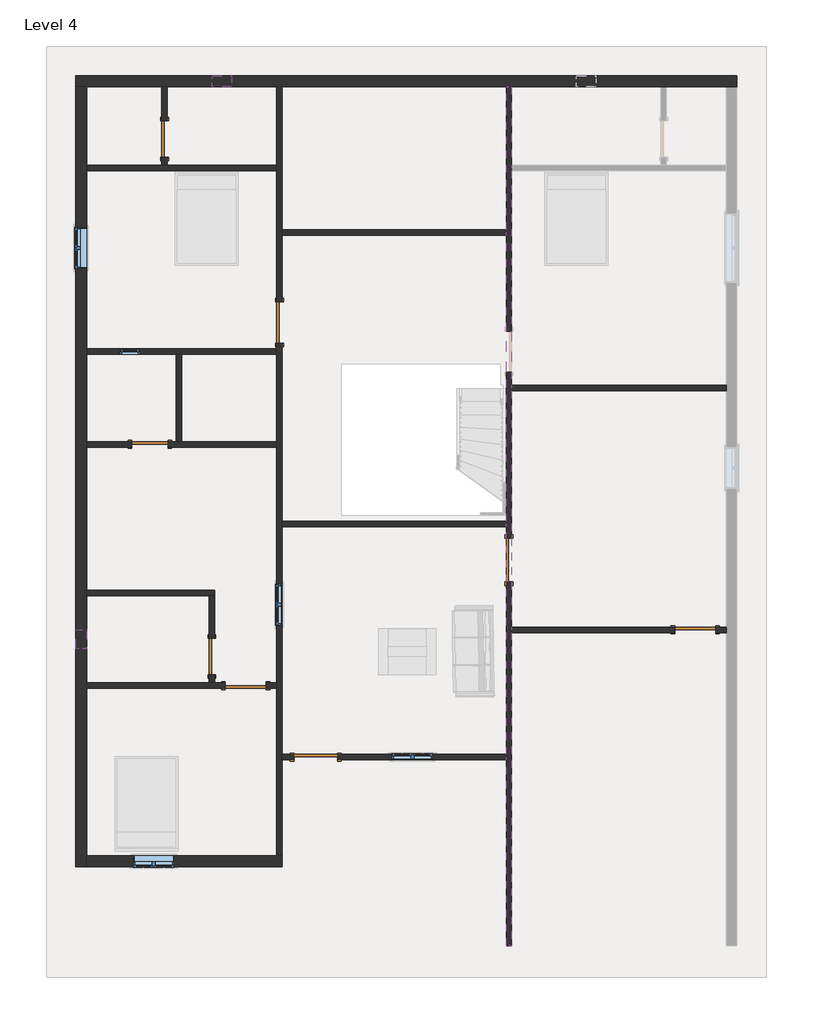
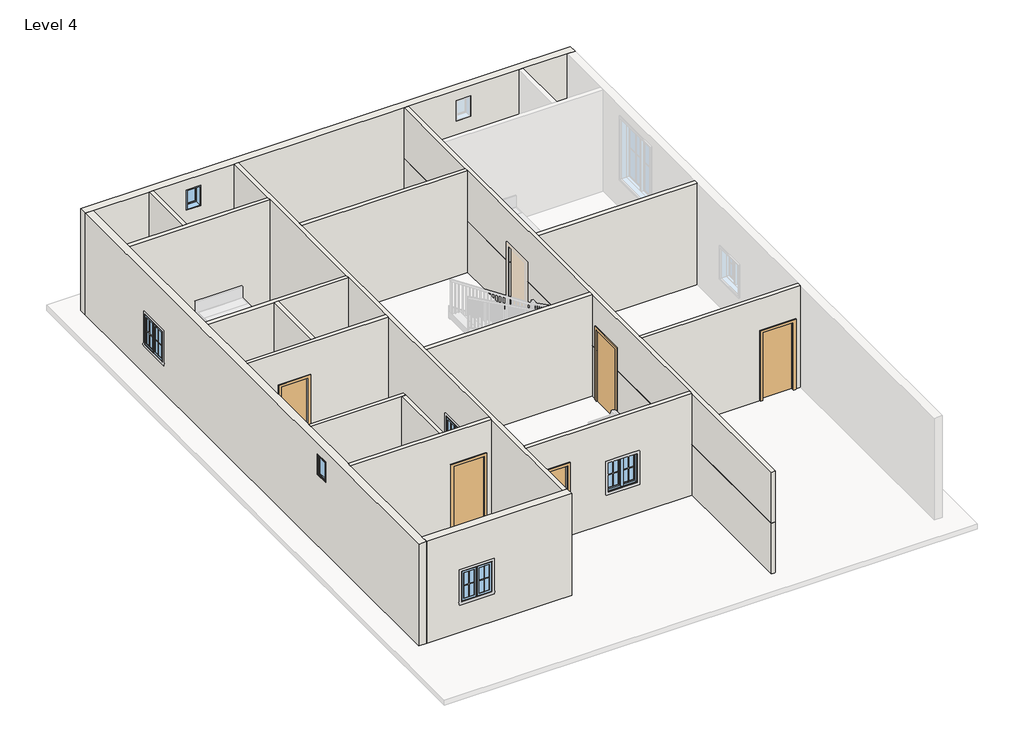
# One storey, part 1 of 3: 19 walls, 8 doors, 7 windows.
"""IFC4 building model written with IfcOpenShell, lengths in millimetres."""

from ifc_helpers import new_model, si_unit, frame, origin, place, context, project, spatial, polyline, outline, extrude, faceted_brep, transform, mapped, element, save
from components import door_f2b275c1, door_d8f5dbb5, door_825b8444, door_c29894e6, door_305aa2a5, window_aa618e30, window_a10b4202, window_339605e1, window_a598f463

model = new_model("IFC4")

# Units and contexts
model_context = context("Model", 3, world=origin())
ifc_project = project(units=[si_unit("LENGTHUNIT", "METRE", prefix="MILLI")], contexts=[model_context])

# Site, building, storey
site = spatial("IfcSite", under=ifc_project)
building = spatial("IfcBuilding", under=site)
storey = spatial("IfcBuildingStorey", under=building, Name="Level 4", Elevation=6400.8)

# Doors
placement = place(None, origin())
door_shape = door_f2b275c1(model_context)
element("IfcDoor", 1, ObjectType="Single-Flush : 30\" x 80\"", at=placement, inside=storey, context=model_context, shape_type="MappedRepresentation", body=[
    mapped(door_shape, transform((-5639.8561469, 9100.7522623, 6400.8), x_axis=(0.0, -1.0, 0.0), y_axis=(1.0, 0.0, 0.0), z_axis=(0.0, 0.0, 1.0))),
])
element("IfcDoor", 2, ObjectType="Single-Flush : 30\" x 80\"", at=placement, inside=storey, context=model_context, shape_type="MappedRepresentation", body=[
    mapped(door_shape, transform((-4646.033646, -1745.0477377, 6400.8), x_axis=(0.0, -1.0, 0.0), y_axis=(1.0, 0.0, 0.0), z_axis=(0.0, 0.0, 1.0))),
])
door_2_shape = door_d8f5dbb5(model_context)
element("IfcDoor", 3, ObjectType="Single-Flush : 30\" x 80\"", at=placement, inside=storey, context=model_context, shape_type="MappedRepresentation", body=[
    mapped(door_2_shape, transform((-5947.8915084, 2699.9522623, 6400.8), x_axis=(1.0, 0.0, 0.0), y_axis=(0.0, 1.0, 0.0), z_axis=(0.0, 0.0, 1.0))),
])
door_3_shape = door_825b8444(model_context)
element("IfcDoor", 4, ObjectType="Single-Flush : 34\" x 80\"", at=placement, inside=storey, context=model_context, shape_type="MappedRepresentation", body=[
    mapped(door_3_shape, transform((-3230.0915084, 5252.6522623, 6400.8), x_axis=(0.0, -1.0, 0.0), y_axis=(1.0, 0.0, 0.0), z_axis=(0.0, 0.0, 1.0))),
])
element("IfcDoor", 5, ObjectType="Single-Flush : 34\" x 80\"", at=placement, inside=storey, context=model_context, shape_type="MappedRepresentation", body=[
    mapped(door_3_shape, transform((-3938.0625772, -2354.6477377, 6400.8), x_axis=(1.0, 0.0, 0.0), y_axis=(0.0, 1.0, 0.0), z_axis=(0.0, 0.0, 1.0))),
])
door_4_shape = door_c29894e6(model_context)
element("IfcDoor", 6, ObjectType="Single-Flush : 34\" x 80\"", at=placement, inside=storey, context=model_context, shape_type="MappedRepresentation", body=[
    mapped(door_4_shape, transform((5488.4584916, -1186.2477377, 6400.8), x_axis=(1.0, 0.0, 0.0), y_axis=(0.0, 1.0, 0.0), z_axis=(0.0, 0.0, 1.0))),
])
door_5_shape = door_305aa2a5(model_context)
element("IfcDoor", 7, ObjectType="Single-Flush : 36\" x 84\"", at=placement, inside=storey, context=model_context, shape_type="MappedRepresentation", body=[
    mapped(door_5_shape, transform((1583.2084916, 274.2522623, 6400.8), x_axis=(0.0, -1.0, 0.0), y_axis=(1.0, 0.0, 0.0), z_axis=(0.0, 0.0, 1.0))),
])
element("IfcDoor", 8, ObjectType="Single-Flush : 36\" x 84\"", at=placement, inside=storey, context=model_context, shape_type="MappedRepresentation", body=[
    mapped(door_5_shape, transform((-2468.0915084, -3853.2477377, 6400.8), x_axis=(-1.0, 0.0, 0.0), y_axis=(0.0, -1.0, 0.0), z_axis=(0.0, 0.0, 1.0))),
])

# Walls
element("IfcWall", 9, ObjectType="9\"", at=placement, inside=storey, context=model_context, shape_type="Brep", body=[
    faceted_brep([(-7503.6415084, 10199.3022623, 6400.8), (-7275.0415084, 10199.3022623, 6400.8), (-5697.0061469, 10199.3022623, 6400.8), (-5582.7061469, 10199.3022623, 6400.8), (-3287.2415084, 10199.3022623, 6400.8), (-3172.9415084, 10199.3022623, 6400.8), (1526.0584916, 10199.3022623, 6400.8), (1640.3584916, 10199.3022623, 6400.8), (4770.1866507, 10199.3022623, 6400.8), (4884.4866507, 10199.3022623, 6400.8), (6136.1584916, 10199.3022623, 6400.8), (6364.7584916, 10199.3022623, 6400.8), (6364.7584916, 10199.3022623, 9448.8), (6136.1584916, 10199.3022623, 9448.8), (4884.4866507, 10199.3022623, 9448.8), (4770.1866507, 10199.3022623, 9448.8), (1640.3584916, 10199.3022623, 9448.8), (1526.0584916, 10199.3022623, 9448.8), (-3172.9415084, 10199.3022623, 9448.8), (-3287.2415084, 10199.3022623, 9448.8), (-5582.7061469, 10199.3022623, 9448.8), (-5697.0061469, 10199.3022623, 9448.8), (-7275.0415084, 10199.3022623, 9448.8), (-7503.6415084, 10199.3022623, 9448.8), (-4231.7738276, 10199.3022623, 9144.0), (-4231.7738276, 10199.3022623, 8534.4), (-4638.1738276, 10199.3022623, 8534.4), (-4638.1738276, 10199.3022623, 9144.0), (3408.4725711, 10199.3022623, 9144.0), (3408.4725711, 10199.3022623, 8534.4), (3002.0725711, 10199.3022623, 8534.4), (3002.0725711, 10199.3022623, 9144.0), (-7503.6415084, 10427.9022623, 6400.8), (-7503.6415084, 10427.9022623, 9448.8), (6364.7584916, 10427.9022623, 9448.8), (6364.7584916, 10427.9022623, 6400.8), (-4231.7738276, 10427.9022623, 9144.0), (-4638.1738276, 10427.9022623, 9144.0), (-4638.1738276, 10427.9022623, 8534.4), (-4231.7738276, 10427.9022623, 8534.4), (3408.4725711, 10427.9022623, 9144.0), (3002.0725711, 10427.9022623, 9144.0), (3002.0725711, 10427.9022623, 8534.4), (3408.4725711, 10427.9022623, 8534.4)], [[[0, 1, 2, 3, 4, 5, 6, 7, 8, 9, 10, 11, 12, 13, 14, 15, 16, 17, 18, 19, 20, 21, 22, 23], [24, 25, 26, 27], [28, 29, 30, 31]], [[32, 33, 34, 35], [36, 37, 38, 39], [40, 41, 42, 43]], [[11, 10, 9, 8, 7, 6, 5, 4, 3, 2, 1, 0, 32, 35]], [[12, 11, 35, 34]], [[25, 24, 36, 39]], [[26, 25, 39, 38]], [[27, 26, 38, 37]], [[24, 27, 37, 36]], [[29, 28, 40, 43]], [[30, 29, 43, 42]], [[31, 30, 42, 41]], [[28, 31, 41, 40]], [[23, 22, 21, 20, 19, 18, 17, 16, 15, 14, 13, 12, 34, 33]], [[0, 23, 33, 32]]]),
])
element("IfcWall", 10, ObjectType="9\"", at=placement, inside=storey, context=model_context, shape_type="Brep", body=[
    faceted_brep([(-7503.6415084, 10199.3022623, 6400.8), (-7503.6415084, -6145.5977377, 6400.8), (-7503.6415084, -6145.5977377, 9448.8), (-7503.6415084, 10199.3022623, 9448.8), (-7503.6415084, -1179.8977377, 9144.0), (-7503.6415084, -1586.2977377, 9144.0), (-7503.6415084, -1586.2977377, 8534.4), (-7503.6415084, -1179.8977377, 8534.4), (-7503.6415084, 7246.5522623, 8229.6), (-7503.6415084, 6382.9522623, 8229.6), (-7503.6415084, 6382.9522623, 7315.2), (-7503.6415084, 7246.5522623, 7315.2), (-7275.0415084, 10199.3022623, 6400.8), (-7275.0415084, 10199.3022623, 9448.8), (-7275.0415084, 8548.3022623, 9448.8), (-7275.0415084, 8434.0022623, 9448.8), (-7275.0415084, 4700.2022623, 9448.8), (-7275.0415084, 4585.9022623, 9448.8), (-7275.0415084, 2757.1022623, 9448.8), (-7275.0415084, 2642.8022623, 9448.8), (-7275.0415084, -354.3977377, 9448.8), (-7275.0415084, -468.6977377, 9448.8), (-7275.0415084, -2297.4977377, 9448.8), (-7275.0415084, -2411.7977377, 9448.8), (-7275.0415084, -5916.9977377, 9448.8), (-7275.0415084, -6145.5977377, 9448.8), (-7275.0415084, -6145.5977377, 6400.8), (-7275.0415084, -5916.9977377, 6400.8), (-7275.0415084, -2411.7977377, 6400.8), (-7275.0415084, -2297.4977377, 6400.8), (-7275.0415084, -468.6977377, 6400.8), (-7275.0415084, -354.3977377, 6400.8), (-7275.0415084, 2642.8022623, 6400.8), (-7275.0415084, 2757.1022623, 6400.8), (-7275.0415084, 4585.9022623, 6400.8), (-7275.0415084, 4700.2022623, 6400.8), (-7275.0415084, 8434.0022623, 6400.8), (-7275.0415084, 8548.3022623, 6400.8), (-7275.0415084, -1179.8977377, 9144.0), (-7275.0415084, -1179.8977377, 8534.4), (-7275.0415084, -1586.2977377, 8534.4), (-7275.0415084, -1586.2977377, 9144.0), (-7275.0415084, 7246.5522623, 8229.6), (-7275.0415084, 7246.5522623, 7315.2), (-7275.0415084, 6382.9522623, 7315.2), (-7275.0415084, 6382.9522623, 8229.6)], [[[0, 1, 2, 3], [4, 5, 6, 7], [8, 9, 10, 11]], [[12, 13, 14, 15, 16, 17, 18, 19, 20, 21, 22, 23, 24, 25, 26, 27, 28, 29, 30, 31, 32, 33, 34, 35, 36, 37], [38, 39, 40, 41], [42, 43, 44, 45]], [[1, 0, 12, 37, 36, 35, 34, 33, 32, 31, 30, 29, 28, 27, 26]], [[2, 1, 26, 25]], [[39, 38, 4, 7]], [[40, 39, 7, 6]], [[41, 40, 6, 5]], [[38, 41, 5, 4]], [[43, 42, 8, 11]], [[44, 43, 11, 10]], [[45, 44, 10, 9]], [[42, 45, 9, 8]], [[3, 2, 25, 24, 23, 22, 21, 20, 19, 18, 17, 16, 15, 14, 13]], [[0, 3, 13, 12]]]),
])
element("IfcWall", 11, ObjectType="9\"", at=placement, inside=storey, context=model_context, shape_type="Brep", body=[
    faceted_brep([(-7275.0415084, -6145.5977377, 6400.8), (-3172.9415084, -6145.5977377, 6400.8), (-3172.9415084, -6145.5977377, 9448.8), (-7275.0415084, -6145.5977377, 9448.8), (-6297.1415084, -6145.5977377, 8229.6), (-5433.5415084, -6145.5977377, 8229.6), (-5433.5415084, -6145.5977377, 7315.2), (-6297.1415084, -6145.5977377, 7315.2), (-7275.0415084, -5916.9977377, 6400.8), (-7275.0415084, -5916.9977377, 9448.8), (-3287.2415084, -5916.9977377, 9448.8), (-3172.9415084, -5916.9977377, 9448.8), (-3172.9415084, -5916.9977377, 6400.8), (-3287.2415084, -5916.9977377, 6400.8), (-6297.1415084, -5916.9977377, 8229.6), (-6297.1415084, -5916.9977377, 7315.2), (-5433.5415084, -5916.9977377, 7315.2), (-5433.5415084, -5916.9977377, 8229.6)], [[[0, 1, 2, 3], [4, 5, 6, 7]], [[8, 9, 10, 11, 12, 13], [14, 15, 16, 17]], [[1, 0, 8, 13, 12]], [[0, 3, 9, 8]], [[2, 1, 12, 11]], [[15, 14, 4, 7]], [[16, 15, 7, 6]], [[17, 16, 6, 5]], [[14, 17, 5, 4]], [[3, 2, 11, 10, 9]]]),
])
element("IfcWall", 12, ObjectType="WALL4.5\"", at=placement, inside=storey, context=model_context, shape_type="Brep", body=[
    faceted_brep([(-7275.0415084, 8434.0022623, 6400.8), (-3287.2415084, 8434.0022623, 6400.8), (-3287.2415084, 8434.0022623, 9448.8), (-7275.0415084, 8434.0022623, 9448.8), (-7275.0415084, 8548.3022623, 6400.8), (-7275.0415084, 8548.3022623, 9448.8), (-5697.0061469, 8548.3022623, 9448.8), (-5582.7061469, 8548.3022623, 9448.8), (-3287.2415084, 8548.3022623, 9448.8), (-3287.2415084, 8548.3022623, 6400.8), (-5582.7061469, 8548.3022623, 6400.8), (-5697.0061469, 8548.3022623, 6400.8)], [[[0, 1, 2, 3]], [[4, 5, 6, 7, 8, 9, 10, 11]], [[1, 0, 4, 11, 10, 9]], [[0, 3, 5, 4]], [[2, 1, 9, 8]], [[3, 2, 8, 7, 6, 5]]]),
])
element("IfcWall", 13, ObjectType="WALL4.5\"", at=placement, inside=storey, context=model_context, shape_type="SweptSolid", body=[
    extrude(outline(polyline([(8719.7522623, 8432.8), (8719.7522623, 6400.8), (8548.3022623, 6400.8), (8548.3022623, 9448.8), (10199.3022623, 9448.8), (10199.3022623, 6400.8), (9481.7522623, 6400.8), (9481.7522623, 8432.8), (8719.7522623, 8432.8)])), frame((-5697.0061469, 0.0, 0.0), z_axis=(1.0, 0.0, 0.0), x_axis=(0.0, 1.0, 0.0)), (0.0, 0.0, 1.0), 114.3),
])
element("IfcWall", 14, ObjectType="WALL4.5\"", at=placement, inside=storey, context=model_context, shape_type="Brep", body=[
    faceted_brep([(-3287.2415084, 4820.8522623, 8432.8), (-3287.2415084, 4820.8522623, 6400.8), (-3287.2415084, 4700.2022623, 6400.8), (-3287.2415084, 4585.9022623, 6400.8), (-3287.2415084, 2757.1022623, 6400.8), (-3287.2415084, 2642.8022623, 6400.8), (-3287.2415084, -2297.4977377, 6400.8), (-3287.2415084, -2411.7977377, 6400.8), (-3287.2415084, -5916.9977377, 6400.8), (-3287.2415084, -5916.9977377, 9448.8), (-3287.2415084, -2411.7977377, 9448.8), (-3287.2415084, -2297.4977377, 9448.8), (-3287.2415084, 2642.8022623, 9448.8), (-3287.2415084, 2757.1022623, 9448.8), (-3287.2415084, 4585.9022623, 9448.8), (-3287.2415084, 4700.2022623, 9448.8), (-3287.2415084, 8434.0022623, 9448.8), (-3287.2415084, 8548.3022623, 9448.8), (-3287.2415084, 10199.3022623, 9448.8), (-3287.2415084, 10199.3022623, 6400.8), (-3287.2415084, 8548.3022623, 6400.8), (-3287.2415084, 8434.0022623, 6400.8), (-3287.2415084, 5684.4522623, 6400.8), (-3287.2415084, 5684.4522623, 8432.8), (-3287.2415084, -227.3977377, 8229.6), (-3287.2415084, -1090.9977377, 8229.6), (-3287.2415084, -1090.9977377, 7315.2), (-3287.2415084, -227.3977377, 7315.2), (-3172.9415084, -5916.9977377, 6400.8), (-3172.9415084, -3910.3977377, 6400.8), (-3172.9415084, -3796.0977377, 6400.8), (-3172.9415084, 979.1022623, 6400.8), (-3172.9415084, 1093.4022623, 6400.8), (-3172.9415084, 4820.8522623, 6400.8), (-3172.9415084, 4820.8522623, 8432.8), (-3172.9415084, 5684.4522623, 8432.8), (-3172.9415084, 5684.4522623, 6400.8), (-3172.9415084, 7087.8022623, 6400.8), (-3172.9415084, 7202.1022623, 6400.8), (-3172.9415084, 10199.3022623, 6400.8), (-3172.9415084, 10199.3022623, 9448.8), (-3172.9415084, 7202.1022623, 9448.8), (-3172.9415084, 7087.8022623, 9448.8), (-3172.9415084, 1093.4022623, 9448.8), (-3172.9415084, 979.1022623, 9448.8), (-3172.9415084, -3796.0977377, 9448.8), (-3172.9415084, -3910.3977377, 9448.8), (-3172.9415084, -5916.9977377, 9448.8), (-3172.9415084, -227.3977377, 8229.6), (-3172.9415084, -227.3977377, 7315.2), (-3172.9415084, -1090.9977377, 7315.2), (-3172.9415084, -1090.9977377, 8229.6)], [[[0, 1, 2, 3, 4, 5, 6, 7, 8, 9, 10, 11, 12, 13, 14, 15, 16, 17, 18, 19, 20, 21, 22, 23], [24, 25, 26, 27]], [[28, 29, 30, 31, 32, 33, 34, 35, 36, 37, 38, 39, 40, 41, 42, 43, 44, 45, 46, 47], [48, 49, 50, 51]], [[22, 21, 20, 19, 39, 38, 37, 36]], [[8, 7, 6, 5, 4, 3, 2, 1, 33, 32, 31, 30, 29, 28]], [[9, 8, 28, 47]], [[19, 18, 40, 39]], [[34, 33, 1, 0]], [[35, 34, 0, 23]], [[36, 35, 23, 22]], [[49, 48, 24, 27]], [[50, 49, 27, 26]], [[51, 50, 26, 25]], [[48, 51, 25, 24]], [[18, 17, 16, 15, 14, 13, 12, 11, 10, 9, 47, 46, 45, 44, 43, 42, 41, 40]]]),
])
element("IfcWall", 15, ObjectType="WALL4.5\"", at=placement, inside=storey, context=model_context, shape_type="Brep", body=[
    faceted_brep([(-7275.0415084, 4585.9022623, 6400.8), (-5395.4415084, 4585.9022623, 6400.8), (-5281.1415084, 4585.9022623, 6400.8), (-3287.2415084, 4585.9022623, 6400.8), (-3287.2415084, 4585.9022623, 9448.8), (-5281.1415084, 4585.9022623, 9448.8), (-5395.4415084, 4585.9022623, 9448.8), (-7275.0415084, 4585.9022623, 9448.8), (-6160.6165084, 4585.9022623, 7924.8), (-6160.6165084, 4585.9022623, 7315.2), (-6567.0165084, 4585.9022623, 7315.2), (-6567.0165084, 4585.9022623, 7924.8), (-7275.0415084, 4700.2022623, 6400.8), (-7275.0415084, 4700.2022623, 9448.8), (-3287.2415084, 4700.2022623, 9448.8), (-3287.2415084, 4700.2022623, 6400.8), (-6160.6165084, 4700.2022623, 7924.8), (-6567.0165084, 4700.2022623, 7924.8), (-6567.0165084, 4700.2022623, 7315.2), (-6160.6165084, 4700.2022623, 7315.2)], [[[0, 1, 2, 3, 4, 5, 6, 7], [8, 9, 10, 11]], [[12, 13, 14, 15], [16, 17, 18, 19]], [[3, 2, 1, 0, 12, 15]], [[0, 7, 13, 12]], [[4, 3, 15, 14]], [[9, 8, 16, 19]], [[10, 9, 19, 18]], [[11, 10, 18, 17]], [[8, 11, 17, 16]], [[7, 6, 5, 4, 14, 13]]]),
])
element("IfcWall", 16, ObjectType="WALL4.5\"", at=placement, inside=storey, context=model_context, shape_type="SweptSolid", body=[
    extrude(outline(polyline([(-5395.4415084, 2757.1022623), (-5395.4415084, 4585.9022623), (-5281.1415084, 4585.9022623), (-5281.1415084, 2757.1022623), (-5395.4415084, 2757.1022623)])), frame((0.0, 0.0, 6400.8), z_axis=(0.0, 0.0, 1.0), x_axis=(1.0, 0.0, 0.0)), (0.0, 0.0, 1.0), 3048.0),
])
element("IfcWall", 17, ObjectType="WALL4.5\"", at=placement, inside=storey, context=model_context, shape_type="Brep", body=[
    faceted_brep([(-5566.8915084, 2642.8022623, 8432.8), (-5566.8915084, 2642.8022623, 6400.8), (-3287.2415084, 2642.8022623, 6400.8), (-3287.2415084, 2642.8022623, 9448.8), (-7275.0415084, 2642.8022623, 9448.8), (-7275.0415084, 2642.8022623, 6400.8), (-6328.8915084, 2642.8022623, 6400.8), (-6328.8915084, 2642.8022623, 8432.8), (-3287.2415084, 2757.1022623, 6400.8), (-5281.1415084, 2757.1022623, 6400.8), (-5395.4415084, 2757.1022623, 6400.8), (-5566.8915084, 2757.1022623, 6400.8), (-5566.8915084, 2757.1022623, 8432.8), (-6328.8915084, 2757.1022623, 8432.8), (-6328.8915084, 2757.1022623, 6400.8), (-7275.0415084, 2757.1022623, 6400.8), (-7275.0415084, 2757.1022623, 9448.8), (-5395.4415084, 2757.1022623, 9448.8), (-5281.1415084, 2757.1022623, 9448.8), (-3287.2415084, 2757.1022623, 9448.8)], [[[0, 1, 2, 3, 4, 5, 6, 7]], [[8, 9, 10, 11, 12, 13, 14, 15, 16, 17, 18, 19]], [[6, 5, 15, 14]], [[2, 1, 11, 10, 9, 8]], [[5, 4, 16, 15]], [[3, 2, 8, 19]], [[12, 11, 1, 0]], [[13, 12, 0, 7]], [[14, 13, 7, 6]], [[4, 3, 19, 18, 17, 16]]]),
])
element("IfcWall", 18, ObjectType="WALL4.5\"", at=placement, inside=storey, context=model_context, shape_type="Brep", body=[
    faceted_brep([(-7275.0415084, -468.6977377, 6400.8), (-4703.183646, -468.6977377, 6400.8), (-4588.883646, -468.6977377, 6400.8), (-4588.883646, -468.6977377, 9448.8), (-4703.183646, -468.6977377, 9448.8), (-7275.0415084, -468.6977377, 9448.8), (-7275.0415084, -354.3977377, 6400.8), (-7275.0415084, -354.3977377, 9448.8), (-4588.883646, -354.3977377, 9448.8), (-4588.883646, -354.3977377, 6400.8)], [[[0, 1, 2, 3, 4, 5]], [[6, 7, 8, 9]], [[2, 1, 0, 6, 9]], [[0, 5, 7, 6]], [[3, 2, 9, 8]], [[5, 4, 3, 8, 7]]]),
])
element("IfcWall", 19, ObjectType="WALL4.5\"", at=placement, inside=storey, context=model_context, shape_type="SweptSolid", body=[
    extrude(outline(polyline([(-2126.0477377, 8432.8), (-2126.0477377, 6400.8), (-2297.4977377, 6400.8), (-2297.4977377, 9448.8), (-468.6977377, 9448.8), (-468.6977377, 6400.8), (-1364.0477377, 6400.8), (-1364.0477377, 8432.8), (-2126.0477377, 8432.8)])), frame((-4703.183646, 0.0, 0.0), z_axis=(1.0, 0.0, 0.0), x_axis=(0.0, 1.0, 0.0)), (0.0, 0.0, 1.0), 114.3),
])
element("IfcWall", 20, ObjectType="WALL4.5\"", at=placement, inside=storey, context=model_context, shape_type="Brep", body=[
    faceted_brep([(-3506.2625772, -2411.7977377, 8432.8), (-3506.2625772, -2411.7977377, 6400.8), (-3287.2415084, -2411.7977377, 6400.8), (-3287.2415084, -2411.7977377, 9448.8), (-7275.0415084, -2411.7977377, 9448.8), (-7275.0415084, -2411.7977377, 6400.8), (-4369.8625772, -2411.7977377, 6400.8), (-4369.8625772, -2411.7977377, 8432.8), (-3287.2415084, -2297.4977377, 6400.8), (-3506.2625772, -2297.4977377, 6400.8), (-3506.2625772, -2297.4977377, 8432.8), (-4369.8625772, -2297.4977377, 8432.8), (-4369.8625772, -2297.4977377, 6400.8), (-4588.883646, -2297.4977377, 6400.8), (-4703.183646, -2297.4977377, 6400.8), (-7275.0415084, -2297.4977377, 6400.8), (-7275.0415084, -2297.4977377, 9448.8), (-4703.183646, -2297.4977377, 9448.8), (-4588.883646, -2297.4977377, 9448.8), (-3287.2415084, -2297.4977377, 9448.8)], [[[0, 1, 2, 3, 4, 5, 6, 7]], [[8, 9, 10, 11, 12, 13, 14, 15, 16, 17, 18, 19]], [[6, 5, 15, 14, 13, 12]], [[2, 1, 9, 8]], [[5, 4, 16, 15]], [[3, 2, 8, 19]], [[10, 9, 1, 0]], [[11, 10, 0, 7]], [[12, 11, 7, 6]], [[4, 3, 19, 18, 17, 16]]]),
])
element("IfcWall", 21, ObjectType="WALL4.5\"", at=placement, inside=storey, context=model_context, shape_type="SweptSolid", body=[
    extrude(outline(polyline([(1526.0584916, 7087.8022623), (-3172.9415084, 7087.8022623), (-3172.9415084, 7202.1022623), (1526.0584916, 7202.1022623), (1526.0584916, 7087.8022623)])), frame((0.0, 0.0, 6400.8), z_axis=(0.0, 0.0, 1.0), x_axis=(1.0, 0.0, 0.0)), (0.0, 0.0, 1.0), 3048.0),
])
element("IfcWall", 22, ObjectType="WALL4.5\"", at=placement, inside=storey, context=model_context, shape_type="Brep", body=[
    faceted_brep([(1526.0584916, -7802.9477377, 6400.8), (1526.0584916, -7802.9477377, 7924.8), (1526.0584916, -182.9477377, 7924.8), (1526.0584916, -182.9477377, 6400.8), (1526.0584916, -3796.0977377, 6400.8), (1526.0584916, -3910.3977377, 6400.8), (1640.3584916, -7802.9477377, 7924.8), (1640.3584916, -7802.9477377, 6400.8), (1640.3584916, -1243.3977377, 6400.8), (1640.3584916, -1129.0977377, 6400.8), (1640.3584916, -182.9477377, 6400.8), (1640.3584916, -182.9477377, 7924.8)], [[[0, 1, 2, 3, 4, 5]], [[6, 7, 8, 9, 10, 11]], [[7, 0, 5, 4, 3, 10, 9, 8]], [[1, 0, 7, 6]], [[1, 6, 11, 2]], [[3, 2, 11, 10]]]),
    faceted_brep([(1526.0584916, 10199.3022623, 7924.8), (1526.0584916, 10199.3022623, 6400.8), (1526.0584916, 7202.1022623, 6400.8), (1526.0584916, 7087.8022623, 6400.8), (1526.0584916, 5074.8522623, 6400.8), (1526.0584916, 5074.8522623, 7924.8), (1640.3584916, 10199.3022623, 6400.8), (1640.3584916, 10199.3022623, 7924.8), (1640.3584916, 5074.8522623, 7924.8), (1640.3584916, 5074.8522623, 6400.8), (1640.3584916, 8434.0022623, 6400.8), (1640.3584916, 8548.3022623, 6400.8)], [[[0, 1, 2, 3, 4, 5]], [[6, 7, 8, 9, 10, 11]], [[1, 6, 11, 10, 9, 4, 3, 2]], [[7, 0, 5, 8]], [[1, 0, 7, 6]], [[5, 4, 9, 8]]]),
    faceted_brep([(1526.0584916, 4211.2522623, 7924.8), (1526.0584916, 4211.2522623, 6400.8), (1526.0584916, 1093.4022623, 6400.8), (1526.0584916, 979.1022623, 6400.8), (1526.0584916, 731.4522623, 6400.8), (1526.0584916, 731.4522623, 7924.8), (1640.3584916, 4211.2522623, 6400.8), (1640.3584916, 4211.2522623, 7924.8), (1640.3584916, 731.4522623, 7924.8), (1640.3584916, 731.4522623, 6400.8), (1640.3584916, 3823.9022623, 6400.8), (1640.3584916, 3938.2022623, 6400.8)], [[[0, 1, 2, 3, 4, 5]], [[6, 7, 8, 9, 10, 11]], [[1, 6, 11, 10, 9, 4, 3, 2]], [[7, 0, 5, 8]], [[1, 0, 7, 6]], [[5, 4, 9, 8]]]),
])
element("IfcWall", 23, ObjectType="WALL4.5\"", at=placement, inside=storey, context=model_context, shape_type="SweptSolid", body=[
    extrude(outline(polyline([(6400.8, -3172.9415084), (6400.8, -2925.2915084), (8534.4, -2925.2915084), (8534.4, -2010.8915084), (6400.8, -2010.8915084), (6400.8, 1526.0584916), (9448.8, 1526.0584916), (9448.8, -3172.9415084), (6400.8, -3172.9415084)]), holes=[polyline([(8229.6, -10.6415084), (7315.2, -10.6415084), (7315.2, -874.2415084), (8229.6, -874.2415084), (8229.6, -10.6415084)])]), frame((0.0, -3910.3977377, 0.0), z_axis=(0.0, 1.0, 0.0), x_axis=(0.0, 0.0, 1.0)), (0.0, 0.0, 1.0), 114.3),
])
element("IfcWall", 24, ObjectType="WALL4.5\"", at=placement, inside=storey, context=model_context, shape_type="SweptSolid", body=[
    extrude(outline(polyline([(1526.0584916, 979.1022623), (-3172.9415084, 979.1022623), (-3172.9415084, 1093.4022623), (1526.0584916, 1093.4022623), (1526.0584916, 979.1022623)])), frame((0.0, 0.0, 6400.8), z_axis=(0.0, 0.0, 1.0), x_axis=(1.0, 0.0, 0.0)), (0.0, 0.0, 1.0), 3048.0),
])
element("IfcWall", 25, ObjectType="WALL4.5\"", at=placement, inside=storey, context=model_context, shape_type="SweptSolid", body=[
    extrude(outline(polyline([(6136.1584916, 3823.9022623), (1640.3584916, 3823.9022623), (1640.3584916, 3938.2022623), (6136.1584916, 3938.2022623), (6136.1584916, 3823.9022623)])), frame((0.0, 0.0, 6400.8), z_axis=(0.0, 0.0, 1.0), x_axis=(1.0, 0.0, 0.0)), (0.0, 0.0, 1.0), 3048.0),
])
element("IfcWall", 26, ObjectType="WALL4.5\"", at=placement, inside=storey, context=model_context, shape_type="SweptSolid", body=[
    extrude(outline(polyline([(8432.8, 5920.2584916), (6400.8, 5920.2584916), (6400.8, 6136.1584916), (9448.8, 6136.1584916), (9448.8, 1640.3584916), (6400.8, 1640.3584916), (6400.8, 5056.6584916), (8432.8, 5056.6584916), (8432.8, 5920.2584916)])), frame((0.0, -1243.3977377, 0.0), z_axis=(0.0, 1.0, 0.0), x_axis=(0.0, 0.0, 1.0)), (0.0, 0.0, 1.0), 114.3),
])
element("IfcWall", 27, ObjectType="WALL4.5\"", at=placement, inside=storey, context=model_context, shape_type="Brep", body=[
    faceted_brep([(1526.0584916, -7802.9477377, 7924.8), (1526.0584916, -7802.9477377, 9448.8), (1526.0584916, -3910.3977377, 9448.8), (1526.0584916, -3796.0977377, 9448.8), (1526.0584916, 979.1022623, 9448.8), (1526.0584916, 1093.4022623, 9448.8), (1526.0584916, 7087.8022623, 9448.8), (1526.0584916, 7202.1022623, 9448.8), (1526.0584916, 10199.3022623, 9448.8), (1526.0584916, 10199.3022623, 7924.8), (1526.0584916, 5074.8522623, 7924.8), (1526.0584916, 5074.8522623, 8432.8), (1526.0584916, 4211.2522623, 8432.8), (1526.0584916, 4211.2522623, 7924.8), (1526.0584916, 731.4522623, 7924.8), (1526.0584916, 731.4522623, 8534.4), (1526.0584916, -182.9477377, 8534.4), (1526.0584916, -182.9477377, 7924.8), (1640.3584916, -7802.9477377, 9448.8), (1640.3584916, -7802.9477377, 7924.8), (1640.3584916, -182.9477377, 7924.8), (1640.3584916, -182.9477377, 8534.4), (1640.3584916, 731.4522623, 8534.4), (1640.3584916, 731.4522623, 7924.8), (1640.3584916, 4211.2522623, 7924.8), (1640.3584916, 4211.2522623, 8432.8), (1640.3584916, 5074.8522623, 8432.8), (1640.3584916, 5074.8522623, 7924.8), (1640.3584916, 10199.3022623, 7924.8), (1640.3584916, 10199.3022623, 9448.8), (1640.3584916, 8548.3022623, 9448.8), (1640.3584916, 8434.0022623, 9448.8), (1640.3584916, 3938.2022623, 9448.8), (1640.3584916, 3823.9022623, 9448.8), (1640.3584916, -1129.0977377, 9448.8), (1640.3584916, -1243.3977377, 9448.8)], [[[0, 1, 2, 3, 4, 5, 6, 7, 8, 9, 10, 11, 12, 13, 14, 15, 16, 17]], [[18, 19, 20, 21, 22, 23, 24, 25, 26, 27, 28, 29, 30, 31, 32, 33, 34, 35]], [[19, 0, 17, 20]], [[13, 24, 23, 14]], [[10, 9, 28, 27]], [[1, 0, 19, 18]], [[12, 25, 24, 13]], [[25, 12, 11, 26]], [[26, 11, 10, 27]], [[16, 21, 20, 17]], [[21, 16, 15, 22]], [[22, 15, 14, 23]], [[9, 8, 29, 28]], [[8, 7, 6, 5, 4, 3, 2, 1, 18, 35, 34, 33, 32, 31, 30, 29]]]),
])

# Windows
window_shape = window_aa618e30(model_context)
element("IfcWindow", 28, ObjectType="Fixed : 16\" x 24\"", at=placement, inside=storey, context=model_context, shape_type="MappedRepresentation", body=[
    mapped(window_shape, transform((-4396.8738276, 10313.6022623, 7620.0), x_axis=(1.0, 0.0, 0.0), y_axis=(0.0, 1.0, 0.0), z_axis=(0.0, 0.0, 1.0))),
])
element("IfcWindow", 29, ObjectType="Fixed : 16\" x 24\"", at=placement, inside=storey, context=model_context, shape_type="MappedRepresentation", body=[
    mapped(window_shape, transform((-7389.3415084, -1344.9977377, 7620.0), x_axis=(0.0, 1.0, 0.0), y_axis=(-1.0, 0.0, 0.0), z_axis=(0.0, 0.0, 1.0))),
])
window_2_shape = window_a10b4202(model_context)
element("IfcWindow", 30, ObjectType="Fixed : 16\" x 24\"", at=placement, inside=storey, context=model_context, shape_type="MappedRepresentation", body=[
    mapped(window_2_shape, transform((-6325.7165084, 4643.0522623, 6400.8), x_axis=(1.0, 0.0, 0.0), y_axis=(0.0, 1.0, 0.0), z_axis=(0.0, 0.0, 1.0))),
])
window_3_shape = window_339605e1(model_context)
element("IfcWindow", 31, ObjectType="Window-Casement-Double : 34\" x 36\"", at=placement, inside=storey, context=model_context, shape_type="MappedRepresentation", body=[
    mapped(window_3_shape, transform((-7389.3415084, 6814.7522623, 6400.8), x_axis=(0.0, 1.0, 0.0), y_axis=(-1.0, 0.0, 0.0), z_axis=(0.0, 0.0, 1.0))),
])
element("IfcWindow", 32, ObjectType="Window-Casement-Double : 34\" x 36\"", at=placement, inside=storey, context=model_context, shape_type="MappedRepresentation", body=[
    mapped(window_3_shape, transform((-5865.3415084, -6031.2977377, 6400.8), x_axis=(-1.0, 0.0, 0.0), y_axis=(0.0, -1.0, 0.0), z_axis=(0.0, 0.0, 1.0))),
])
window_4_shape = window_a598f463(model_context)
element("IfcWindow", 33, ObjectType="Window-Casement-Double : 34\" x 36\"", at=placement, inside=storey, context=model_context, shape_type="MappedRepresentation", body=[
    mapped(window_4_shape, transform((-442.4415084, -3853.2477377, 6400.8), x_axis=(1.0, 0.0, 0.0), y_axis=(0.0, 1.0, 0.0), z_axis=(0.0, 0.0, 1.0))),
])
element("IfcWindow", 34, ObjectType="Window-Casement-Double : 34\" x 36\"", at=placement, inside=storey, context=model_context, shape_type="MappedRepresentation", body=[
    mapped(window_4_shape, transform((-3230.0915084, -659.1977377, 6400.8), x_axis=(0.0, 1.0, 0.0), y_axis=(-1.0, 0.0, 0.0), z_axis=(0.0, 0.0, 1.0))),
])

save(model, "model.ifc")

# Revit data of these elements
# Type "Single-Flush : 30\" x 80\""
#   Type Mark = "5"
#   Construction Type Id = "MDOOR"
#   Assembly Code = "C1020"
#   Analytic Construction = "Metal"
#   Thickness = 0' - 2"
#   Heat Transfer Coefficient (U) = 0.651978 BTU/(h·ft²·°F)
#   Height = 6' - 8"
#   Trim Projection Ext = 0' - 1"
#   Trim Projection Int = 0' - 1"
#   Trim Width = 0' - 3"
#   Width = 2' - 6"
#   Define Thermal Properties by = 1
#   Define Thermal Properties by = 1
#   Door Material = Door - Panel
#   Frame Material = Door - Frame
#   Visual Light Transmittance = 0
#   Solar Heat Gain Coefficient = 0
#   Function = (empty or 0)
#   Wall Closure = (empty or 0)
# Type "Single-Flush : 34\" x 80\""
#   Type Mark = "7"
#   Construction Type Id = "MDOOR"
#   Assembly Code = "C1020"
#   Analytic Construction = "Metal"
#   Thickness = 0' - 2"
#   Heat Transfer Coefficient (U) = 0.651978 BTU/(h·ft²·°F)
#   Height = 6' - 8"
#   Trim Projection Ext = 0' - 1"
#   Trim Projection Int = 0' - 1"
#   Trim Width = 0' - 3"
#   Width = 2' - 10"
#   Define Thermal Properties by = 1
#   Define Thermal Properties by = 1
#   Door Material = Door - Panel
#   Frame Material = Door - Frame
#   Visual Light Transmittance = 0
#   Solar Heat Gain Coefficient = 0
#   Function = (empty or 0)
#   Wall Closure = (empty or 0)
# Type "Single-Flush : 36\" x 84\""
#   Type Mark = "1"
#   Construction Type Id = "MDOOR"
#   Assembly Code = "C1020"
#   Analytic Construction = "Metal"
#   Thickness = 0' - 2"
#   Heat Transfer Coefficient (U) = 0.651978 BTU/(h·ft²·°F)
#   Height = 7' - 0"
#   Trim Projection Ext = 0' - 1"
#   Trim Projection Int = 0' - 1"
#   Trim Width = 0' - 3"
#   Width = 3' - 0"
#   Define Thermal Properties by = 1
#   Define Thermal Properties by = 1
#   Door Material = Door - Panel
#   Frame Material = Door - Frame
#   Visual Light Transmittance = 0
#   Solar Heat Gain Coefficient = 0
#   Function = (empty or 0)
#   Wall Closure = (empty or 0)
# Type "9\""
#   Assembly Code = "B2010"
#   Layers, outside or top first: 0' - 9" no material (function 1)
# Type "WALL4.5\""
#   Assembly Code = "B2010"
#   Layers, outside or top first: 0' - 4 1/2" no material (function 1)
# Type "Fixed : 16\" x 24\""
#   Type Mark = "4"
#   Construction Type Id = "GSP4R"
#   Assembly Code = "B2020100"
#   Analytic Construction = "1/8 in Pilkington single glazing"
#   Visual Light Transmittance = 0.9
#   Solar Heat Gain Coefficient = 0.78
#   Heat Transfer Coefficient (U) = 0.6496 BTU/(h·ft²·°F)
#   Height = 2' - 0"
#   Default Sill Height = 3' - 0"
#   Width = 1' - 4"
#   Window Inset = 0' - 0 3/4"
#   Define Thermal Properties by = 1
#   Define Thermal Properties by = 1
#   Glass Pane Material = Glass
#   Sash Material = Sash
#   Wall Closure = (empty or 0)
# Type "Window-Casement-Double : 34\" x 36\""
#   Type Mark = "14"
#   Fire Rating = "0.5h"
#   Assembly Code = "B2020100"
#   Analytic Construction = "Double glazing - domestic"
#   Frame Extension [instance default] = 0' - 0 1/4"
#   Window Inset [instance default] = 0' - 0"
#   Wall Thickness [instance default] = 0' - 6"
#   Interior Wall Closure [instance default] = 0' - 2 1/4"
#   Half Width = 1' - 5"
#   Visual Light Transmittance = 0.81
#   Thermal Resistance (R) = 1.8146 (h·ft²·°F)/BTU
#   Solar Heat Gain Coefficient = 0.76
#   Rough Width = 2' - 10 1/2"
#   Rough Height = 3' - 0 1/2"
#   Height = 3' - 0"
#   Heat Transfer Coefficient (U) = 0.5511 BTU/(h·ft²·°F)
#   Exterior Wall Closure [instance default] = 0' - 1 1/4"
#   Extension Jamb [instance default] = 0' - 2 1/4"
#   Default Sill Height = 3' - 0"
#   Width = 2' - 10"
#   Define Thermal Properties by = 0
#   Muntin Visibility = yes
#   Interior Trim Visibility [instance default] = yes
#   Exterior Trim Visibility [instance default] = yes
#   Extension Jamb Visibility [instance default] = yes
#   Interior Trim Material = Wood - Stained
#   Muntin Pattern = Muntin Pattern_2x2 : Muntin Pattern_2x2
#   Interior Trim = Trim-Window-Interior-Flat : Picture Frame
#   Interior Frame Material = Wood - Stained
#   Glass Panel Material = Glass
#   Exterior Trim Material = Clad - White
#   Exterior Trim = Trim-Window-Exterior-Flat : with Sill
#   Exterior Frame Material = Clad - White
#   Wall Closure = (empty or 0)
# Elements 1, 2, 3 (IfcDoor, "Single-Flush : 30\" x 80\"")
#   Phase Created = New Construction
#   Materials on its faces: "Door - Frame", "Door - Panel"
# Elements 4, 5, 6 (IfcDoor, "Single-Flush : 34\" x 80\"")
#   Phase Created = New Construction
#   Materials on its faces: "Door - Frame", "Door - Panel"
# Elements 7, 8 (IfcDoor, "Single-Flush : 36\" x 84\"")
#   Phase Created = New Construction
#   Materials on its faces: "Door - Frame", "Door - Panel"
# Elements 9, 10, 11 (IfcWall, "9\"")
#   Top Offset = 0' - 0"
#   Base Offset = 0' - 0"
#   Unconnected Height = 10' - 0"
#   wall height = 10' - 0"
#   Phase Created = New Construction
#   Base Constraint = Level 4
#   Materials on its faces: "Default Wall", "legs"
# Elements 12, 13, 15, 16, 17, 18, 19, 21, 24, 25 (IfcWall, "WALL4.5\"")
#   Top Offset = 0' - 0"
#   Base Offset = 0' - 0"
#   Unconnected Height = 10' - 0"
#   wall height = 10' - 0"
#   Phase Created = New Construction
#   Base Constraint = Level 4
#   Materials on its faces: "Default Wall"
# Elements 14, 23, 26 (IfcWall, "WALL4.5\"")
#   Top Offset = 0' - 0"
#   Base Offset = 0' - 0"
#   Unconnected Height = 10' - 0"
#   wall height = 10' - 0"
#   Phase Created = New Construction
#   Base Constraint = Level 4
#   Materials on its faces: "Default Wall", "legs"
# Element 20 (IfcWall, "WALL4.5\"")
#   Top Offset = 0' - 0"
#   Base Offset = 0' - 0"
#   Unconnected Height = 10' - 0"
#   wall height = 10' - 0"
#   Phase Created = New Construction
#   Base Constraint = Level 4
#   Materials on its faces: "Default Wall", "Wood and Glass Coffee Table - Wood"
# Element 22 (IfcWall, "WALL4.5\"")
#   Top Offset = 0' - 0"
#   Base Offset = 0' - 0"
#   Unconnected Height = 5' - 0"
#   wall height = 5' - 0"
#   Phase Created = New Construction
#   Base Constraint = Level 4
#   Materials on its faces: "Default Wall", "legs"
# Element 27 (IfcWall, "WALL4.5\"")
#   built-in parameter 1001111 = 5' - 0"
#   Top Offset = 0' - 0"
#   Base Offset = 5' - 0"
#   Unconnected Height = 5' - 0"
#   wall height = 5' - 0"
#   Phase Created = New Construction
#   Base Constraint = Level 4
#   Materials on its faces: "Default Wall", "legs"
# Element 28 (IfcWindow, "Fixed : 16\" x 24\"")
#   Mark = "21"
#   Phase Created = New Construction
#   Materials on its faces: "Sash", "Glass"
# Element 29 (IfcWindow, "Fixed : 16\" x 24\"")
#   Mark = "24"
#   Phase Created = New Construction
#   Materials on its faces: "Sash", "Glass"
# Element 30 (IfcWindow, "Fixed : 16\" x 24\"")
#   Mark = "23"
#   Phase Created = New Construction
#   Materials on its faces: "Sash", "Glass"
# Element 31 (IfcWindow, "Window-Casement-Double : 34\" x 36\"")
#   Mark = "25"
#   Window Inset = 0' - 0"
#   Interior Wall Closure = 0' - 2 1/4"
#   Frame Extension = 0' - 0 1/4"
#   Exterior Wall Closure = 0' - 1 1/4"
#   Interior Trim Visibility = yes
#   Exterior Trim Visibility = yes
#   Phase Created = New Construction
#   Materials on its faces: "Wood - Stained", "Glass", "Clad - White"
# Element 32 (IfcWindow, "Window-Casement-Double : 34\" x 36\"")
#   Mark = "26"
#   Window Inset = 0' - 0"
#   Interior Wall Closure = 0' - 2 1/4"
#   Frame Extension = 0' - 0 1/4"
#   Exterior Wall Closure = 0' - 1 1/4"
#   Interior Trim Visibility = yes
#   Exterior Trim Visibility = yes
#   Phase Created = New Construction
#   Materials on its faces: "Wood - Stained", "Glass", "Clad - White"
# Element 33 (IfcWindow, "Window-Casement-Double : 34\" x 36\"")
#   Mark = "27"
#   Window Inset = 0' - 0"
#   Interior Wall Closure = 0' - 2 1/4"
#   Frame Extension = 0' - 0 1/4"
#   Exterior Wall Closure = 0' - 1 1/4"
#   Interior Trim Visibility = yes
#   Exterior Trim Visibility = yes
#   Phase Created = New Construction
#   Materials on its faces: "Wood - Stained", "Glass", "Clad - White"
# Element 34 (IfcWindow, "Window-Casement-Double : 34\" x 36\"")
#   Mark = "30"
#   Window Inset = 0' - 0"
#   Interior Wall Closure = 0' - 2 1/4"
#   Frame Extension = 0' - 0 1/4"
#   Exterior Wall Closure = 0' - 1 1/4"
#   Interior Trim Visibility = yes
#   Exterior Trim Visibility = yes
#   Phase Created = New Construction
#   Materials on its faces: "Wood - Stained", "Glass", "Clad - White"
# Materials
#   "Door - Panel": class "Wood", colour RGB 210 159 95, transparency 0, Cost = 0
#   "Door - Frame": colour RGB 118 70 51, transparency 0, Cost = 0
#   "Glass": class "Glass", colour RGB 0 128 192, transparency 0.75, Description = "Soda Lime Glass", Cost = 0
#   "Sash": class "Wood", colour RGB 224 178 126, transparency 0, Cost = 0
#   "Wood - Stained": class "Wood", colour RGB 224 178 126, transparency 0, Cost = 0
#   "Clad - White": class "Wood", colour RGB 242 242 238, transparency 0, Cost = 0
#   "Default Wall": colour RGB 128 128 128, transparency 0, Cost = 0
#   "legs": colour RGB 90 73 37, transparency 0, Cost = 0
#   "Wood and Glass Coffee Table - Wood": class "Generic", colour RGB 120 120 120, transparency 0, Cost = 0
